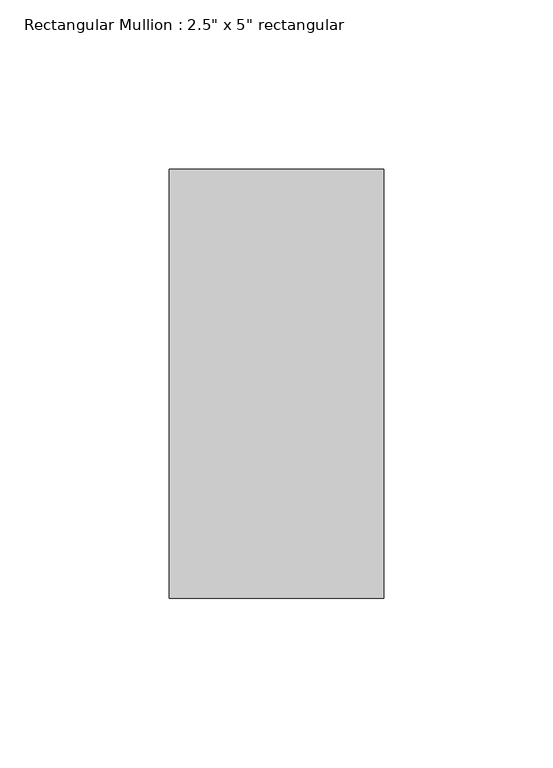
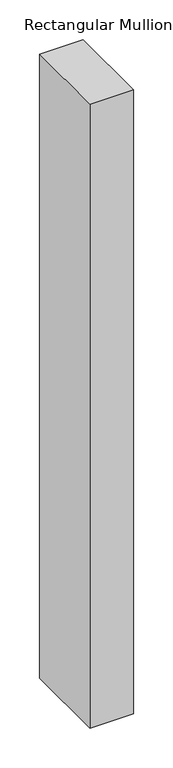
"""IFC4 building model written with IfcOpenShell, lengths in millimetres: member geometry."""

from ifc_helpers import new_model, si_unit, frame, origin, place, context, project, spatial, polyline, outline, extrude, source, transform, mapped, element, save


def member_f8454dad(model_context):
    return source(origin(), model_context, "Body", "SweptSolid", [
        extrude(outline(polyline([(0.0, 63.5), (0.0, -63.5), (-63.5, -63.5), (-63.5, 63.5), (0.0, 63.5)])), frame((0.0, 0.0, -961.0064813), z_axis=(0.0, 0.0, 1.0), x_axis=(1.0, 0.0, 0.0)), (0.0, 0.0, 1.0), 961.0064813),
    ])


if __name__ == "__main__":
    model = new_model("IFC4")
    model_context = context("Model", 3, world=origin())
    ifc_project = project(units=[si_unit("LENGTHUNIT", "METRE", prefix="MILLI")], contexts=[model_context])
    site = spatial("IfcSite", under=ifc_project)
    building = spatial("IfcBuilding", under=site)
    placement = place(None, origin())
    member_shape = member_f8454dad(model_context)
    element("IfcMember", 1, ObjectType="Rectangular Mullion : 2.5\" x 5\" rectangular", at=placement, inside=building, context=model_context, shape_type="MappedRepresentation", body=[
        mapped(member_shape, transform((0.0, 0.0, 0.0), x_axis=(1.0, 0.0, 0.0), y_axis=(0.0, 1.0, 0.0), z_axis=(0.0, 0.0, 1.0))),
    ])
    save(model, "model.ifc")

# Revit data of these elements
# Type "Rectangular Mullion : 2.5\" x 5\" rectangular"
#   built-in parameter 1007304 = 0.416667 (stored number, unit not read)
#   built-in parameter 1007301 = 0.104167 (stored number, unit not read)
#   built-in parameter 1007300 = 0.104167 (stored number, unit not read)
# Element 1 (IfcMember, "Rectangular Mullion : 2.5\" x 5\" rectangular")
#   Materials on its faces: "Aluminum"
# Materials
#   "Aluminum": class "Metal", colour RGB 247 247 247, transparency 0, Description = "Aluminum 6061", Cost = 0
